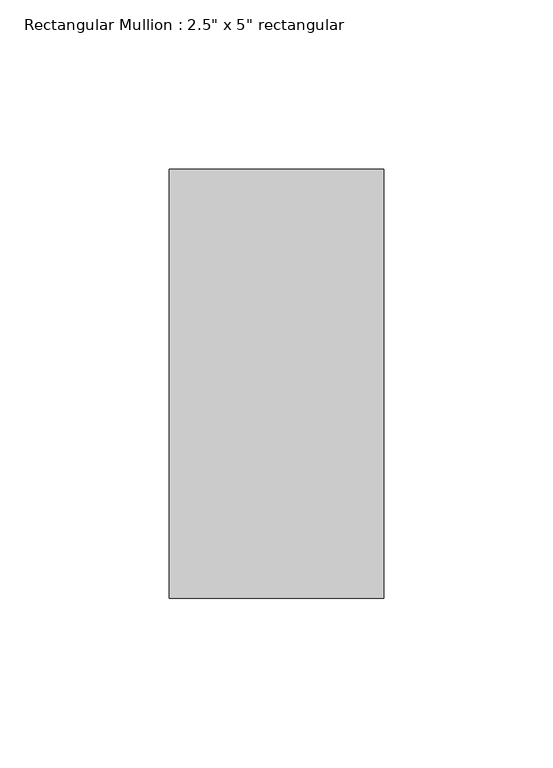
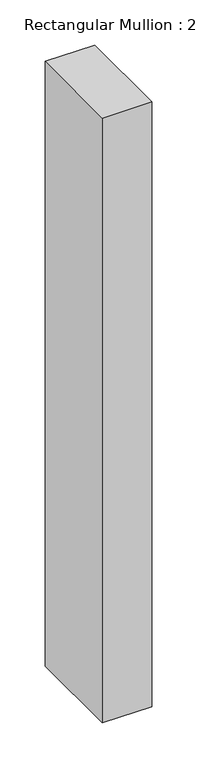
"""IFC4 building model written with IfcOpenShell, lengths in millimetres: member geometry."""

from ifc_helpers import new_model, si_unit, frame, origin, place, context, project, spatial, polyline, outline, extrude, source, transform, mapped, element, save


def member_bef5179f(model_context):
    return source(origin(), model_context, "Body", "SweptSolid", [
        extrude(outline(polyline([(0.0, 63.5), (0.0, -63.5), (-63.5, -63.5), (-63.5, 63.5), (0.0, 63.5)])), frame((0.0, 0.0, -819.1500001), z_axis=(0.0, 0.0, 1.0), x_axis=(1.0, 0.0, 0.0)), (0.0, 0.0, 1.0), 819.1500001),
    ])


if __name__ == "__main__":
    model = new_model("IFC4")
    model_context = context("Model", 3, world=origin())
    ifc_project = project(units=[si_unit("LENGTHUNIT", "METRE", prefix="MILLI")], contexts=[model_context])
    site = spatial("IfcSite", under=ifc_project)
    building = spatial("IfcBuilding", under=site)
    placement = place(None, origin())
    member_shape = member_bef5179f(model_context)
    element("IfcMember", 1, ObjectType="Rectangular Mullion : 2.5\" x 5\" rectangular", at=placement, inside=building, context=model_context, shape_type="MappedRepresentation", body=[
        mapped(member_shape, transform((0.0, 0.0, 0.0), x_axis=(1.0, 0.0, 0.0), y_axis=(0.0, 1.0, 0.0), z_axis=(0.0, 0.0, 1.0))),
    ])
    save(model, "model.ifc")

# Revit data of these elements
# Type "Rectangular Mullion : 2.5\" x 5\" rectangular"
#   built-in parameter 1007304 = 0.416667 (stored number, unit not read)
#   built-in parameter 1007301 = 0.104167 (stored number, unit not read)
#   built-in parameter 1007300 = 0.104167 (stored number, unit not read)
# Element 1 (IfcMember, "Rectangular Mullion : 2.5\" x 5\" rectangular")
#   Materials on its faces: "Aluminum"
# Materials
#   "Aluminum": class "Metal", colour RGB 247 247 247, transparency 0, Description = "Aluminum 6061", Cost = 0
